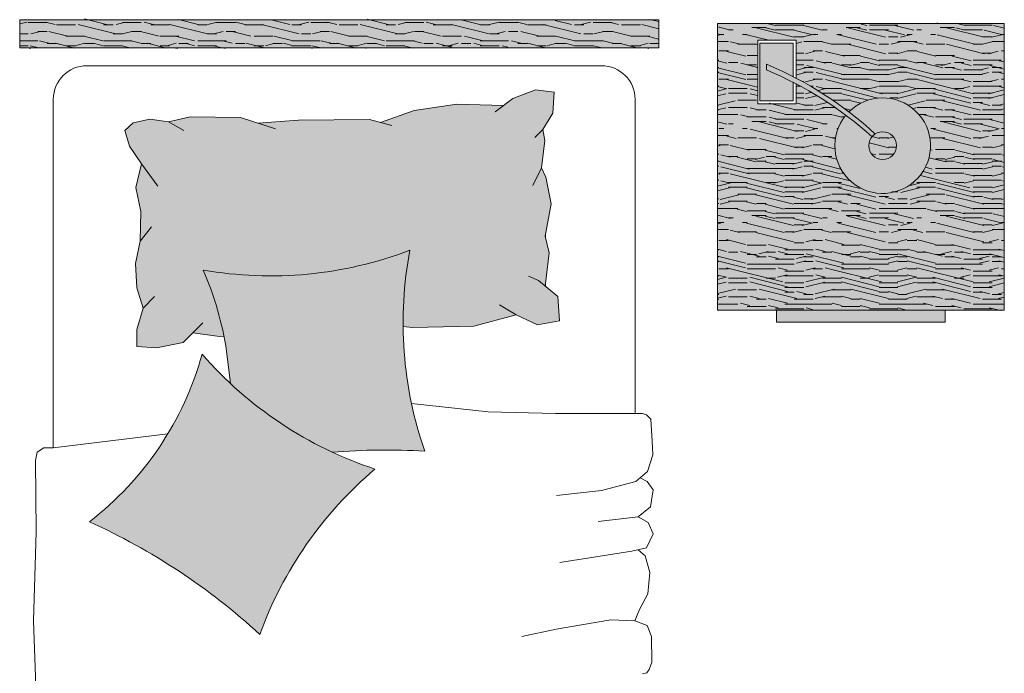
# Model space of a CAD drawing. Units: inches. Extents: x 1994 to 3075, y 3517 to 3950.
# Tile 19 of 58: x 1994.71013 to 1994.76776, y 3553.27657 to 3553.31483. Entities that reach past the tile are written whole.
import ezdxf

# ---------------------------------------------------------------- set-up
doc = ezdxf.new("R2010")
doc.units = ezdxf.units.IN
doc.layers.add('A-FURN-REFR', color=8, linetype='Continuous', lineweight=13)
doc.layers.add('A-FURN-REFR-PATT', color=8, linetype='Continuous', lineweight=13)

msp = doc.modelspace()

# ---------------------------------------------------------------- hatches: boundary and pattern name
at = {"layer": 'A-FURN-REFR-PATT'}
for points in [[(1994.74752711248, 3553.314834833183), (1994.710125537677, 3553.314834833183), (1994.710125537677, 3553.313186285147), (1994.74752711248, 3553.313186285147)], [(1994.755400221191, 3553.313454285159), (1994.753453346297, 3553.313454285159), (1994.753453346297, 3553.310087285902), (1994.755400221191, 3553.310087285902), (1994.755400221191, 3553.311165699976, 0.0198106445216732), (1994.753838065744, 3553.311892743406), (1994.753838065744, 3553.312223669301, -0.0198106445216994), (1994.755400221191, 3553.311496625872), (1994.755400221191, 3553.311503507754)]]:
    msp.add_hatch(color=256, dxfattribs=at).paths.add_polyline_path(points)
h = msp.add_hatch(dxfattribs=at)
h.set_pattern_fill('LEGNO1', color=256, scale=0.005511811023622, style=0, pattern_type=2)
h.set_pattern_definition([(0, (2000.356371596277, 3548.921636491977), (0, 0.005511811023622), [0.0011023622047244, -0.0016535433070866, 0.0005511811023622, -0.0022047244094488]), (0, (2000.360229863994, 3548.921774287253), (0, 0.005511811023622), [0.0011023622047244, -0.0044094488188976]), (0, (2000.359678682892, 3548.922049877804), (0, 0.005511811023622), [0.0005511811023622, -0.0049606299212598]), (0, (2000.356647186829, 3548.92218767308), (0, 0.005511811023622), [0.0002755905511811, -0.0038582677165354, 0.0002755905511811, -0.0011023622047244]), (0, (2000.358576320687, 3548.922463263631), (0, 0.005511811023622), [0.0011023622047244, -0.0016535433070866, 0.0002755905511811, -0.0024803149606299]), (0, (2000.357198367931, 3548.922601058907), (0, 0.005511811023622), [0.0008267716535433, -0.0046850393700787]), (0, (2000.358576320687, 3548.922738854182), (0, 0.005511811023622), [0.0016535433070866, -0.0038582677165354]), (0, (2000.356922777379, 3548.922876649458), (0, 0.005511811023622), [0.0011023622047244, -0.0044094488188976]), (0, (2000.35912750179, 3548.923014444734), (0, 0.005511811023622), [0.002755905511811, -0.002755905511811]), (0, (2000.357473958482, 3548.923290035285), (0, 0.005511811023622), [0.0005511811023622, -0.0016535433070866, 0.0011023622047244, -0.0022047244094488]), (0, (2000.361332226199, 3548.923427830561), (0, 0.005511811023622), [0.0011023622047244, -0.0044094488188976]), (0, (2000.360229863994, 3548.923565625836), (0, 0.005511811023622), [0.0005511811023622, -0.0049606299212598]), (0, (2000.35912750179, 3548.923703421111), (0, 0.005511811023622), [0.0005511811023622, -0.0049606299212598]), (0, (2000.356371596277, 3548.923841216387), (0, 0.005511811023622), [0.0011023622047244, -0.0044094488188976]), (0, (2000.35912750179, 3548.923979011662), (0, 0.005511811023622), [0.0011023622047244, -0.0044094488188976]), (0, (2000.35912750179, 3548.924254602213), (0, 0.005511811023622), [0.0011023622047244, -0.0011023622047244, 0.0011023622047244, -0.0022047244094488]), (0, (2000.358025139584, 3548.924530192765), (0, 0.005511811023622), [0.0005511811023622, -0.002755905511811, 0.0011023622047244, -0.0011023622047244]), (0, (2000.35912750179, 3548.92466798804), (0, 0.005511811023622), [0.0016535433070866, -0.0038582677165354]), (0, (2000.35912750179, 3548.924943578592), (0, 0.005511811023622), [0.0011023622047244, -0.0044094488188976]), (0, (2000.356922777379, 3548.925081373867), (0, 0.005511811023622), [0.0016535433070866, -0.0022047244094488, 0.0005511811023622, -0.0011023622047244]), (0, (2000.356922777379, 3548.925356964419), (0, 0.005511811023622), [0.002755905511811, -0.002755905511811]), (0, (2000.360229863994, 3548.925494759694), (0, 0.005511811023622), [0.0005511811023622, -0.0049606299212598]), (0, (2000.358576320687, 3548.92563255497), (0, 0.005511811023622), [0.0011023622047244, -0.0044094488188976]), (0, (2000.357473958482, 3548.925770350245), (0, 0.005511811023622), [0.0005511811023622, -0.0022047244094488, 0.0005511811023622, -0.0022047244094488]), (0, (2000.356922777379, 3548.925908145521), (0, 0.005511811023622), [0.0005511811023622, -0.0016535433070866, 0.0011023622047244, -0.0022047244094488]), (0, (2000.358025139584, 3548.926045940796), (0, 0.005511811023622), [0.0005511811023622, -0.002755905511811, 0.0005511811023622, -0.0016535433070866]), (0, (2000.35912750179, 3548.926183736072), (0, 0.005511811023622), [0.0016535433070866, -0.0038582677165354]), (0, (2000.356922777379, 3548.926459326623), (0, 0.005511811023622), [0.0011023622047244, -0.0044094488188976]), (0, (2000.359678682892, 3548.926597121898), (0, 0.005511811023622), [0.0005511811023622, -0.0049606299212598]), (0, (2000.360781045096, 3548.926734917174), (0, 0.005511811023622), [0.0005511811023622, -0.0049606299212598]), (14.03624347, (2000.360229863994, 3548.922049877804), (0.0055118110234648, -2.016e-13), [0.0005677165354331, -0.0221580619543307]), (14.03624347, (2000.360781045096, 3548.923290035285), (0.0055118110234648, -2.016e-13), [0.0005677165354331, -0.0221580619543307]), (14.03624347, (2000.360229863994, 3548.926597121898), (0.0055118110234648, -2.016e-13), [0.0005677165354331, -0.0221580619543307]), (14.03624347, (2000.358576320687, 3548.924530192765), (0.0055118110234648, -2.016e-13), [0.0005677165354331, -0.0221580619543307]), (14.03624347, (2000.359678682892, 3548.925356964419), (0.0055118110234648, -2.016e-13), [0.0005677165354331, -0.0221580619543307]), (14.03624347, (2000.360229863994, 3548.924943578592), (0.0055118110234648, -2.016e-13), [0.0005677165354331, -0.0221580619543307]), (14.03624347, (2000.357473958482, 3548.925908145521), (0.0055118110234648, -2.016e-13), [0.0005677165354331, -0.0221580619543307]), (14.03624347, (2000.359678682892, 3548.92563255497), (0.0055118110234648, -2.016e-13), [0.0005677165354331, -0.0221580619543307]), (14.03624347, (2000.360781045096, 3548.923565625836), (0.0055118110234648, -2.016e-13), [0.0011354330708661, -0.0215903454188977]), (14.03624347, (2000.360229863994, 3548.923979011662), (0.0055118110234648, -2.016e-13), [0.0011354330708661, -0.0215903454188977]), (14.03624347, (2000.360229863994, 3548.924254602213), (0.0055118110234648, -2.016e-13), [0.0011354330708661, -0.0215903454188977]), (165.96375653, (2000.358576320687, 3548.922463263631), (-0.0055118110234648, -2.016e-13), [0.0005677165354331, -0.0011354330708661, 0.0005677165354331, -0.0204549123480315]), (165.96375653, (2000.357473958482, 3548.923290035285), (-0.0055118110234648, -2.016e-13), [0.0005677165354331, -0.0221580619543307]), (165.96375653, (2000.357473958482, 3548.925770350245), (-0.0055118110234648, -2.016e-13), [0.0011354330708661, -0.0215903454188977]), (194.03624347, (2000.360229863994, 3548.921774287253), (-0.0055118110234648, 2.016e-13), [0.0005677165354331, -0.0221580619543307]), (345.96375653, (2000.361332226199, 3548.921774287253), (0.0055118110234648, 2.016e-13), [0.0005677165354331, -0.0221580619543307]), (345.96375653, (2000.359678682892, 3548.923703421111), (0.0055118110234648, 2.016e-13), [0.0005677165354331, -0.0221580619543307]), (345.96375653, (2000.360781045096, 3548.92466798804), (0.0055118110234648, 2.016e-13), [0.0005677165354331, -0.0221580619543307]), (345.96375653, (2000.358576320687, 3548.925081373867), (0.0055118110234648, 2.016e-13), [0.0005677165354331, -0.0221580619543307]), (345.96375653, (2000.358025139584, 3548.925770350245), (0.0055118110234648, 2.016e-13), [0.0005677165354331, -0.0221580619543307]), (345.96375653, (2000.358576320687, 3548.926045940796), (0.0055118110234648, 2.016e-13), [0.0005677165354331, -0.0221580619543307]), (345.96375653, (2000.358576320687, 3548.925081373867), (0.0055118110234648, 2.016e-13), [0.0005677165354331, -0.0221580619543307]), (345.96375653, (2000.360229863994, 3548.925908145521), (0.0055118110234648, 2.016e-13), [0.0022708661417323, -0.0204549123480315]), (345.96375653, (2000.356922777379, 3548.92218767308), (0.0055118110234648, 2.016e-13), [0.0022708661417323, -0.0204549123480315]), (345.96375653, (2000.357473958482, 3548.922601058907), (0.0055118110234648, 2.016e-13), [0.0022708661417323, -0.0204549123480315]), (345.96375653, (2000.358025139584, 3548.922876649458), (0.0055118110234648, 2.016e-13), [0.0005677165354331, -0.0011354330708661, 0.0011354330708661, -0.0198871958125984]), (345.96375653, (2000.358025139584, 3548.923290035285), (0.0055118110234648, 2.016e-13), [0.0011354330708661, -0.0011354330708661, 0.0011354330708661, -0.0193194792771654]), (345.96375653, (2000.357473958482, 3548.923841216387), (0.0055118110234648, 2.016e-13), [0.0022708661417323, -0.0204549123480315]), (345.96375653, (2000.356922777379, 3548.924254602213), (0.0055118110234648, 2.016e-13), [0.0022708661417323, -0.0204549123480315]), (345.96375653, (2000.356922777379, 3548.924530192765), (0.0055118110234648, 2.016e-13), [0.0022708661417323, -0.0204549123480315]), (345.96375653, (2000.360781045096, 3548.926183736072), (0.0055118110234648, 2.016e-13), [0.0005677165354331, -0.0221580619543307]), (345.9637675300001, (2000.361332226199, 3548.926734917174), (0.0055118110234647, 1.0583933e-09), [0.0011354330708661, -0.0215903454188977]), (345.9637675300001, (2000.358025139584, 3548.926459326623), (0.0055118110234647, 1.0583933e-09), [0.0011354330708661, -0.0215903454188977]), (345.96375753, (2000.357473958482, 3548.921636491977), (0.0055118110234648, 9.64008e-11), [0.0022708661417323, -0.0204549123480315]), (345.96375753, (2000.360781045096, 3548.925494759694), (0.0055118110234648, 9.64008e-11), [0.0017031496062992, -0.0210226288834646]), (345.96375753, (2000.361332226199, 3548.925081373867), (0.0055118110234648, 9.64008e-11), [0.0034062992125984, -0.0193194792771654])])
h.paths.add_polyline_path([(1994.74752711248, 3553.314834833183), (1994.710125537677, 3553.314834833183), (1994.710125537677, 3553.313186285147), (1994.74752711248, 3553.313186285147)])
h = msp.add_hatch(color=256, dxfattribs=at)
h.paths.add_polyline_path([(1994.76775604609, 3553.314620330361), (1994.750973187446, 3553.314620330361), (1994.750973187446, 3553.297837471717), (1994.76775604609, 3553.297837471717)])
h.paths.add_polyline_path([(1994.758479567912, 3553.309240305821, 0.0395152736214826), (1994.755577209817, 3553.311073603386), (1994.755577209817, 3553.309910077288), (1994.753320605166, 3553.309910077288), (1994.753320605166, 3553.313631493773), (1994.755577209817, 3553.313631493773), (1994.755577209817, 3553.311404529282, -0.042086183498597), (1994.758657689699, 3553.309436525341, -42.19598506439468)], flags=16)
h.paths.add_polyline_path([(1994.759827418463, 3553.30746046484, -1), (1994.761447352029, 3553.30746046484, -1)], flags=0)
h = msp.add_hatch(dxfattribs=at)
h.set_pattern_fill('LEGNO1', color=256, scale=0.005511811023622, style=0, pattern_type=2)
h.set_pattern_definition([(0, (2000.776563016131, 3549.493707209018), (0, 0.005511811023622), [0.0011023622047244, -0.0016535433070866, 0.0005511811023622, -0.0022047244094488]), (0, (2000.780421283847, 3549.493845004293), (0, 0.005511811023622), [0.0011023622047244, -0.0044094488188976]), (0, (2000.779870102745, 3549.494120594844), (0, 0.005511811023622), [0.0005511811023622, -0.0049606299212598]), (0, (2000.776838606682, 3549.49425839012), (0, 0.005511811023622), [0.0002755905511811, -0.0038582677165354, 0.0002755905511811, -0.0011023622047244]), (0, (2000.77876774054, 3549.494533980671), (0, 0.005511811023622), [0.0011023622047244, -0.0016535433070866, 0.0002755905511811, -0.0024803149606299]), (0, (2000.777389787784, 3549.494671775947), (0, 0.005511811023622), [0.0008267716535433, -0.0046850393700787]), (0, (2000.77876774054, 3549.494809571223), (0, 0.005511811023622), [0.0016535433070866, -0.0038582677165354]), (0, (2000.777114197233, 3549.494947366498), (0, 0.005511811023622), [0.0011023622047244, -0.0044094488188976]), (0, (2000.779318921642, 3549.495085161774), (0, 0.005511811023622), [0.002755905511811, -0.002755905511811]), (0, (2000.777665378335, 3549.495360752325), (0, 0.005511811023622), [0.0005511811023622, -0.0016535433070866, 0.0011023622047244, -0.0022047244094488]), (0, (2000.781523646052, 3549.4954985476), (0, 0.005511811023622), [0.0011023622047244, -0.0044094488188976]), (0, (2000.780421283847, 3549.495636342876), (0, 0.005511811023622), [0.0005511811023622, -0.0049606299212598]), (0, (2000.779318921642, 3549.495774138151), (0, 0.005511811023622), [0.0005511811023622, -0.0049606299212598]), (0, (2000.776563016131, 3549.495911933428), (0, 0.005511811023622), [0.0011023622047244, -0.0044094488188976]), (0, (2000.779318921642, 3549.496049728702), (0, 0.005511811023622), [0.0011023622047244, -0.0044094488188976]), (0, (2000.779318921642, 3549.496325319254), (0, 0.005511811023622), [0.0011023622047244, -0.0011023622047244, 0.0011023622047244, -0.0022047244094488]), (0, (2000.778216559438, 3549.496600909805), (0, 0.005511811023622), [0.0005511811023622, -0.002755905511811, 0.0011023622047244, -0.0011023622047244]), (0, (2000.779318921642, 3549.496738705081), (0, 0.005511811023622), [0.0016535433070866, -0.0038582677165354]), (0, (2000.779318921642, 3549.497014295632), (0, 0.005511811023622), [0.0011023622047244, -0.0044094488188976]), (0, (2000.777114197233, 3549.497152090907), (0, 0.005511811023622), [0.0016535433070866, -0.0022047244094488, 0.0005511811023622, -0.0011023622047244]), (0, (2000.777114197233, 3549.497427681459), (0, 0.005511811023622), [0.002755905511811, -0.002755905511811]), (0, (2000.780421283847, 3549.497565476734), (0, 0.005511811023622), [0.0005511811023622, -0.0049606299212598]), (0, (2000.77876774054, 3549.49770327201), (0, 0.005511811023622), [0.0011023622047244, -0.0044094488188976]), (0, (2000.777665378335, 3549.497841067285), (0, 0.005511811023622), [0.0005511811023622, -0.0022047244094488, 0.0005511811023622, -0.0022047244094488]), (0, (2000.777114197233, 3549.497978862561), (0, 0.005511811023622), [0.0005511811023622, -0.0016535433070866, 0.0011023622047244, -0.0022047244094488]), (0, (2000.778216559438, 3549.498116657836), (0, 0.005511811023622), [0.0005511811023622, -0.002755905511811, 0.0005511811023622, -0.0016535433070866]), (0, (2000.779318921642, 3549.498254453112), (0, 0.005511811023622), [0.0016535433070866, -0.0038582677165354]), (0, (2000.777114197233, 3549.498530043663), (0, 0.005511811023622), [0.0011023622047244, -0.0044094488188976]), (0, (2000.779870102745, 3549.498667838939), (0, 0.005511811023622), [0.0005511811023622, -0.0049606299212598]), (0, (2000.78097246495, 3549.498805634215), (0, 0.005511811023622), [0.0005511811023622, -0.0049606299212598]), (14.03624347, (2000.780421283847, 3549.494120594844), (0.0055118110234648, -2.016e-13), [0.0005677165354331, -0.0221580619543307]), (14.03624347, (2000.78097246495, 3549.495360752325), (0.0055118110234648, -2.016e-13), [0.0005677165354331, -0.0221580619543307]), (14.03624347, (2000.780421283847, 3549.498667838939), (0.0055118110234648, -2.016e-13), [0.0005677165354331, -0.0221580619543307]), (14.03624347, (2000.77876774054, 3549.496600909805), (0.0055118110234648, -2.016e-13), [0.0005677165354331, -0.0221580619543307]), (14.03624347, (2000.779870102745, 3549.497427681459), (0.0055118110234648, -2.016e-13), [0.0005677165354331, -0.0221580619543307]), (14.03624347, (2000.780421283847, 3549.497014295632), (0.0055118110234648, -2.016e-13), [0.0005677165354331, -0.0221580619543307]), (14.03624347, (2000.777665378335, 3549.497978862561), (0.0055118110234648, -2.016e-13), [0.0005677165354331, -0.0221580619543307]), (14.03624347, (2000.779870102745, 3549.49770327201), (0.0055118110234648, -2.016e-13), [0.0005677165354331, -0.0221580619543307]), (14.03624347, (2000.78097246495, 3549.495636342876), (0.0055118110234648, -2.016e-13), [0.0011354330708661, -0.0215903454188977]), (14.03624347, (2000.780421283847, 3549.496049728702), (0.0055118110234648, -2.016e-13), [0.0011354330708661, -0.0215903454188977]), (14.03624347, (2000.780421283847, 3549.496325319254), (0.0055118110234648, -2.016e-13), [0.0011354330708661, -0.0215903454188977]), (165.96375653, (2000.77876774054, 3549.494533980671), (-0.0055118110234648, -2.016e-13), [0.0005677165354331, -0.0011354330708661, 0.0005677165354331, -0.0204549123480315]), (165.96375653, (2000.777665378335, 3549.495360752325), (-0.0055118110234648, -2.016e-13), [0.0005677165354331, -0.0221580619543307]), (165.96375653, (2000.777665378335, 3549.497841067285), (-0.0055118110234648, -2.016e-13), [0.0011354330708661, -0.0215903454188977]), (194.03624347, (2000.780421283847, 3549.493845004293), (-0.0055118110234648, 2.016e-13), [0.0005677165354331, -0.0221580619543307]), (345.96375653, (2000.781523646052, 3549.493845004293), (0.0055118110234648, 2.016e-13), [0.0005677165354331, -0.0221580619543307]), (345.96375653, (2000.779870102745, 3549.495774138151), (0.0055118110234648, 2.016e-13), [0.0005677165354331, -0.0221580619543307]), (345.96375653, (2000.78097246495, 3549.496738705081), (0.0055118110234648, 2.016e-13), [0.0005677165354331, -0.0221580619543307]), (345.96375653, (2000.77876774054, 3549.497152090907), (0.0055118110234648, 2.016e-13), [0.0005677165354331, -0.0221580619543307]), (345.96375653, (2000.778216559438, 3549.497841067285), (0.0055118110234648, 2.016e-13), [0.0005677165354331, -0.0221580619543307]), (345.96375653, (2000.77876774054, 3549.498116657836), (0.0055118110234648, 2.016e-13), [0.0005677165354331, -0.0221580619543307]), (345.96375653, (2000.77876774054, 3549.497152090907), (0.0055118110234648, 2.016e-13), [0.0005677165354331, -0.0221580619543307]), (345.96375653, (2000.780421283847, 3549.497978862561), (0.0055118110234648, 2.016e-13), [0.0022708661417323, -0.0204549123480315]), (345.96375653, (2000.777114197233, 3549.49425839012), (0.0055118110234648, 2.016e-13), [0.0022708661417323, -0.0204549123480315]), (345.96375653, (2000.777665378335, 3549.494671775947), (0.0055118110234648, 2.016e-13), [0.0022708661417323, -0.0204549123480315]), (345.96375653, (2000.778216559438, 3549.494947366498), (0.0055118110234648, 2.016e-13), [0.0005677165354331, -0.0011354330708661, 0.0011354330708661, -0.0198871958125984]), (345.96375653, (2000.778216559438, 3549.495360752325), (0.0055118110234648, 2.016e-13), [0.0011354330708661, -0.0011354330708661, 0.0011354330708661, -0.0193194792771654]), (345.96375653, (2000.777665378335, 3549.495911933428), (0.0055118110234648, 2.016e-13), [0.0022708661417323, -0.0204549123480315]), (345.96375653, (2000.777114197233, 3549.496325319254), (0.0055118110234648, 2.016e-13), [0.0022708661417323, -0.0204549123480315]), (345.96375653, (2000.777114197233, 3549.496600909805), (0.0055118110234648, 2.016e-13), [0.0022708661417323, -0.0204549123480315]), (345.96375653, (2000.78097246495, 3549.498254453112), (0.0055118110234648, 2.016e-13), [0.0005677165354331, -0.0221580619543307]), (345.9637675300001, (2000.781523646052, 3549.498805634215), (0.0055118110234647, 1.0583933e-09), [0.0011354330708661, -0.0215903454188977]), (345.9637675300001, (2000.778216559438, 3549.498530043663), (0.0055118110234647, 1.0583933e-09), [0.0011354330708661, -0.0215903454188977]), (345.96375753, (2000.777665378335, 3549.493707209018), (0.0055118110234648, 9.64008e-11), [0.0022708661417323, -0.0204549123480315]), (345.96375753, (2000.78097246495, 3549.497565476734), (0.0055118110234648, 9.64008e-11), [0.0017031496062992, -0.0210226288834646]), (345.96375753, (2000.781523646052, 3549.497152090907), (0.0055118110234648, 9.64008e-11), [0.0034062992125984, -0.0193194792771654])])
h.paths.add_polyline_path([(1994.76775604609, 3553.314620330361), (1994.750973187446, 3553.314620330361), (1994.750973187446, 3553.297837471717), (1994.76775604609, 3553.297837471717)])
h.paths.add_polyline_path([(1994.753320605166, 3553.309910077288), (1994.753320605166, 3553.313631493773), (1994.755577209817, 3553.313631493773), (1994.755577209817, 3553.311404529282, -0.042086183498597), (1994.758657689699, 3553.309436525341, -42.19598506432865), (1994.758479567912, 3553.309240305821, 0.0395152736214861), (1994.755577209817, 3553.311073603386), (1994.755577209817, 3553.309910077288)], flags=16)
h.paths.add_polyline_path([(1994.759827418463, 3553.30746046484, -1), (1994.761447352029, 3553.30746046484, -1)], flags=0)
h = msp.add_hatch(color=256, dxfattribs=at)
h.dxf.hatch_style = 1
h.set_gradient(color1=(167, 169, 175), one_color=1, tint=1)
h.paths.add_polyline_path([(1994.753838065744, 3553.311892743406), (1994.753838065744, 3553.312223669301, -0.0875286051314429), (1994.76019873732, 3553.308141371726, 0.0763380806476787), (1994.760014634205, 3553.307978371522, 0.0846435149619904)])
h = msp.add_hatch(color=256, dxfattribs=at)
h.set_gradient(color1=(223, 184, 155), color2=(248, 239, 232), one_color=1, tint=0.9399999976158142, name='SPHERICAL')
edge = h.paths.add_edge_path()
edge.add_ellipse((1994.724813374119, 3553.322745777475), major_axis=(-0.0162394621936465, 0.0161586354510627), ratio=0.9999999999999754, start_angle=124.93165070209781, end_angle=155.6980503708569, ccw=False)
edge.add_ellipse((1994.703806775848, 3553.292701605456), major_axis=(0.0131369998350938, 0.013202712122942), ratio=0.9999999999990169, start_angle=326.0032218548852, end_angle=338.5294090826841, ccw=False)
edge.add_line((1994.722080502796, 3553.296302060358), (1994.721824171691, 3553.29628022039))
edge.add_line((1994.721824171691, 3553.29628022039), (1994.720265573822, 3553.296506067916))
edge.add_line((1994.720265573822, 3553.296506067916), (1994.719692777913, 3553.295935777522))
edge.add_line((1994.719692777912, 3553.295935777522), (1994.718133224533, 3553.295626048687))
edge.add_line((1994.718133224533, 3553.295626048687), (1994.716980872298, 3553.29569946425))
edge.add_line((1994.716980872298, 3553.29569946425), (1994.716991652343, 3553.296703707926))
edge.add_line((1994.716991652343, 3553.296703707926), (1994.717346825471, 3553.297943913479))
edge.add_line((1994.717346825471, 3553.29794391348), (1994.716987198101, 3553.299140726493))
edge.add_line((1994.716987198101, 3553.299140726492), (1994.716900483803, 3553.300569161474))
edge.add_line((1994.716900483803, 3553.300569161474), (1994.717179841152, 3553.301876449751))
edge.add_line((1994.717179841153, 3553.301876449751), (1994.717218744079, 3553.303599250499))
edge.add_line((1994.717218744079, 3553.303599250499), (1994.716917589632, 3553.305014667718))
edge.add_line((1994.716917589632, 3553.305014667718), (1994.717264091322, 3553.3063977169))
edge.add_line((1994.717264091322, 3553.3063977169), (1994.71655573514, 3553.307429990013))
edge.add_line((1994.71655573514, 3553.307429990013), (1994.716284930695, 3553.308345455022))
edge.add_line((1994.716284930695, 3553.308345455022), (1994.716759276751, 3553.30880436036))
edge.add_line((1994.716759276751, 3553.308804360361), (1994.717751326011, 3553.309007953546))
edge.add_line((1994.717751326011, 3553.309007953546), (1994.718836533334, 3553.308858777043))
edge.add_line((1994.718836533334, 3553.308858777043), (1994.720110166515, 3553.309151148862))
edge.add_line((1994.720110166515, 3553.309151148862), (1994.723053855134, 3553.309114792965))
edge.add_line((1994.723053855134, 3553.309114792965), (1994.724070921565, 3553.308785153716))
edge.add_line((1994.724070921565, 3553.308785153716), (1994.72643509492, 3553.308961628929))
edge.add_line((1994.72643509492, 3553.308961628929), (1994.730593944388, 3553.308999040351))
edge.add_line((1994.730593944387, 3553.308999040351), (1994.731250378423, 3553.308823799849))
edge.add_line((1994.731250378423, 3553.308823799849), (1994.733217026507, 3553.309516701592))
edge.add_line((1994.733217026506, 3553.309516701592), (1994.735705820534, 3553.309882840731))
edge.add_line((1994.735705820534, 3553.309882840731), (1994.738447054648, 3553.30981764357))
edge.add_line((1994.738447054649, 3553.30981764357), (1994.738985230838, 3553.310225289685))
edge.add_line((1994.738985230838, 3553.310225289685), (1994.740317336921, 3553.310736266038))
edge.add_line((1994.740317336921, 3553.310736266038), (1994.741402544245, 3553.310587089535))
edge.add_line((1994.741402544245, 3553.310587089535), (1994.741333291296, 3553.309364241325))
edge.add_line((1994.741333291296, 3553.309364241325), (1994.740746335734, 3553.308396704976))
edge.add_line((1994.740746335734, 3553.308396704975), (1994.740856837224, 3553.307758248389))
edge.add_line((1994.740856837224, 3553.307758248389), (1994.74066630276, 3553.306169612763))
edge.add_line((1994.74066630276, 3553.306169612762), (1994.740915428641, 3553.305611256336))
edge.add_line((1994.740915428641, 3553.305611256336), (1994.741225254526, 3553.304052995487))
edge.add_line((1994.741225254526, 3553.304052995488), (1994.740888795057, 3553.302153237223))
edge.add_line((1994.740888795058, 3553.302153237223), (1994.741112762962, 3553.301178767854))
edge.add_line((1994.741112762962, 3553.301178767853), (1994.740891792206, 3553.299235319621))
edge.add_line((1994.740891792206, 3553.299235319622), (1994.741626248971, 3553.298629280765))
edge.add_line((1994.741626248971, 3553.298629280765), (1994.741712963269, 3553.297200845783))
edge.add_line((1994.741712963269, 3553.297200845783), (1994.740434993809, 3553.296979895581))
edge.add_line((1994.740434993809, 3553.296979895581), (1994.739180812092, 3553.297548924135))
edge.add_line((1994.739180812092, 3553.297548924135), (1994.73670936092, 3553.296897098066))
edge.add_line((1994.73670936092, 3553.296897098066), (1994.733126688151, 3553.296822978733))
edge.add_line((1994.733126688151, 3553.296822978733), (1994.73256889776, 3553.29686572429))
edge.add_ellipse((1994.755545523121, 3553.297088097322), major_axis=(0.0162071033392254, 0.0162881725219294), ratio=0.9999999999997861, start_angle=124.2042415032482, end_angle=135.411563179048, ccw=False)
h = msp.add_hatch(color=256, dxfattribs=at)
h.dxf.hatch_style = 1
h.set_gradient(color1=(37, 53, 157), color2=(142, 207, 230), tint=1, name='SPHERICAL')
h.paths.add_polyline_path([(1994.760637385246, 3553.308270431623, 0.1440580758931676), (1994.76019873732, 3553.308141371726, 0.0231477939795123), (1994.758657689699, 3553.309436525341, -42.19598506439846), (1994.758479567912, 3553.309240305821, -0.0228504078660832), (1994.760014634205, 3553.307978371522, 0.6355278128427492), (1994.760637385246, 3553.306650498058, 1)])
h = msp.add_hatch(color=256, dxfattribs=at)
h.dxf.hatch_style = 1
h.set_gradient(color1=(37, 40, 142), tint=1, name='INVSPHERICAL')
h.paths.add_polyline_path([(1994.760637385246, 3553.306650498058, -1), (1994.760637385246, 3553.308270431623, -1)])
h = msp.add_hatch(color=256, dxfattribs=at)
h.set_gradient(color1=(216, 161, 105), color2=(246, 232, 219), one_color=1, tint=0.9100000262260437, name='SPHERICAL')
edge = h.paths.add_edge_path()
edge.add_ellipse((1994.738091277294, 3553.310284112182), major_axis=(-0.0162394621936562, 0.0161586354510724), ratio=0.9999999999995159, start_angle=91.86790391008537, end_angle=109.9005060978115, ccw=False)
edge.add_line((1994.722470558145, 3553.293526583568), (1994.722230916878, 3553.295429864856))
edge.add_ellipse((1994.703806775848, 3553.292701605456), major_axis=(-0.0132027121229715, 0.0131369998351231), ratio=0.9999999999985743, start_angle=233.2802454111125, end_angle=248.5294090826748)
edge.add_ellipse((1994.724813374119, 3553.322745777475), major_axis=(-0.0162394621936476, 0.0161586354510638), ratio=0.9999999999999643, start_angle=124.9316507020978, end_angle=155.6980503708595)
edge.add_ellipse((1994.755545523121, 3553.297088097322), major_axis=(0.0162071033392156, 0.0162881725219195), ratio=0.9999999999999907, start_angle=124.2042415032435, end_angle=153.9185959955232)
edge.add_line((1994.733827726711, 3553.289583959675), (1994.733816342417, 3553.289572575381))
edge.add_ellipse((1994.731531269729, 3553.251646479053), major_axis=(-0.026933374560409, 0.0267993222804413), ratio=0.9999999999999866, start_angle=-48.5908820798409, end_angle=-40.45389875014118)
h = msp.add_hatch(color=256, dxfattribs=at)
h.set_gradient(color1=(158, 155, 166), rotation=89.99999999999996, one_color=1, tint=1)
h.paths.add_polyline_path([(1994.764302349481, 3553.297837471717), (1994.754426884055, 3553.297837471717), (1994.754426884055, 3553.297131545392), (1994.764302349481, 3553.297131545392)])
h = msp.add_hatch(color=256, dxfattribs=at)
h.set_gradient(color1=(216, 161, 105), color2=(246, 232, 219), one_color=1, tint=0.9100000262260437, name='SPHERICAL')
edge = h.paths.add_edge_path()
edge.add_ellipse((1994.738091277294, 3553.310284112182), major_axis=(-0.0162394621936485, 0.0161586354510647), ratio=0.9999999999999784, start_angle=85.852665878386, end_angle=116.6190655471458)
edge.add_ellipse((1994.745773584699, 3553.270993353904), major_axis=(0.016207103339218, 0.0162881725219219), ratio=0.9999999999998035, start_angle=85.12525667954132, end_angle=114.8721443105295)
edge.add_ellipse((1994.698485863071, 3553.250856412228), major_axis=(-0.0269333745604207, 0.026799322280453), ratio=0.9999999999996999, start_angle=-87.69350806299315, end_angle=-69.58500463641445)
edge.add_ellipse((1994.702844744636, 3553.300203865216), major_axis=(0.0131369998350991, 0.0132027121229474), ratio=0.9999999999998083, start_angle=262.4507864490607, end_angle=299.4504242589634)

# ---------------------------------------------------------------- linework, layer by layer
at = {"layer": 'A-FURN-REFR'}
for p, q in [((1994.710125537677, 3553.313186285147), (1994.710125537677, 3553.314834833183)), ((1994.74752711248, 3553.314834833183), (1994.710125537677, 3553.314834833183)), ((1994.74752711248, 3553.313186285147), (1994.74752711248, 3553.314834833183)), ((1994.76775604609, 3553.314620330361), (1994.750973187446, 3553.314620330361)), ((1994.750973187446, 3553.314620330361), (1994.750973187446, 3553.297837471717)), ((1994.76775604609, 3553.297837471717), (1994.76775604609, 3553.314620330361)), ((1994.710125537677, 3553.313186285147), (1994.74752711248, 3553.313186285147)), ((1994.753838065744, 3553.312223669301), (1994.753838065744, 3553.311892743406)), ((1994.714062545551, 3553.312143118972), (1994.721377585873, 3553.312143118972)), ((1994.721377585873, 3553.312143118972), (1994.744176183505, 3553.312143118972)), ((1994.740317336921, 3553.310736266038), (1994.738985230838, 3553.310225289685)), ((1994.741402544245, 3553.310587089535), (1994.740317336921, 3553.310736266038)), ((1994.741333291296, 3553.309364241325), (1994.741402544245, 3553.310587089535)), ((1994.712094041614, 3553.289770163587), (1994.712094041614, 3553.310174615035)), ((1994.733217026506, 3553.309516701592), (1994.735705820534, 3553.309882840731)), ((1994.735705820534, 3553.309882840731), (1994.738447054649, 3553.30981764357)), ((1994.738985230838, 3553.310225289685), (1994.737956387239, 3553.309445983383)), ((1994.746144687441, 3553.29505004844), (1994.746144687441, 3553.310174615035)), ((1994.731250378423, 3553.308823799849), (1994.733217026506, 3553.309516701592)), ((1994.740746335734, 3553.308396704975), (1994.741333291296, 3553.309364241325)), ((1994.716759276751, 3553.308804360361), (1994.716284930695, 3553.308345455022)), ((1994.717751326011, 3553.309007953546), (1994.716759276751, 3553.308804360361)), ((1994.718836533334, 3553.308858777043), (1994.717751326011, 3553.309007953546)), ((1994.718836533334, 3553.308858777043), (1994.720110166515, 3553.309151148862)), ((1994.718836533334, 3553.308858777043), (1994.719728979664, 3553.308339473903)), ((1994.720110166515, 3553.309151148862), (1994.723053855134, 3553.309114792965)), ((1994.723053855134, 3553.309114792965), (1994.725102988837, 3553.308450652576)), ((1994.724070921565, 3553.308785153716), (1994.72643509492, 3553.308961628929)), ((1994.72643509492, 3553.308961628929), (1994.730593944387, 3553.308999040351)), ((1994.730593944387, 3553.308999040351), (1994.731906599007, 3553.30864861633)), ((1994.716284930695, 3553.308345455022), (1994.71655573514, 3553.307429990013)), ((1994.740271989678, 3553.307937799637), (1994.740746335734, 3553.308396704975)), ((1994.740856837224, 3553.307758248389), (1994.740746335734, 3553.308396704975)), ((1994.74066630276, 3553.306169612762), (1994.740856837224, 3553.307758248389)), ((1994.71655573514, 3553.307429990013), (1994.717264091322, 3553.3063977169)), ((1994.717264091322, 3553.3063977169), (1994.716917589632, 3553.305014667718)), ((1994.717264091322, 3553.3063977169), (1994.718204229958, 3553.305092774257)), ((1994.740155162385, 3553.30513499398), (1994.74066630276, 3553.306169612762)), ((1994.740915428641, 3553.305611256336), (1994.74066630276, 3553.306169612762)), ((1994.741225254526, 3553.304052995488), (1994.740915428641, 3553.305611256336)), ((1994.716917589632, 3553.305014667718), (1994.717218744079, 3553.303599250499)), ((1994.717218744079, 3553.303599250499), (1994.717179841153, 3553.301876449751)), ((1994.740888795058, 3553.302153237223), (1994.741225254526, 3553.304052995488)), ((1994.717846948793, 3553.302705481434), (1994.717179841153, 3553.301876449751)), ((1994.717179841153, 3553.301876449751), (1994.716900483803, 3553.300569161474)), ((1994.741112762962, 3553.301178767853), (1994.740888795058, 3553.302153237223)), ((1994.740907282327, 3553.302072800351), (1994.740907282327, 3553.302257622287)), ((1994.740891792206, 3553.299235319622), (1994.741112762962, 3553.301178767853)), ((1994.716900483803, 3553.300569161474), (1994.716987198101, 3553.299140726492)), ((1994.740493348199, 3553.299564096703), (1994.739904164944, 3553.2998150696)), ((1994.741626248971, 3553.298629280765), (1994.740493348199, 3553.299564096703)), ((1994.716987198101, 3553.299140726492), (1994.717346825471, 3553.29794391348)), ((1994.740907282327, 3553.299222537909), (1994.740907282327, 3553.299371555971)), ((1994.71802260453, 3553.29863010186), (1994.717346825471, 3553.29794391348)), ((1994.741712963269, 3553.297200845783), (1994.741626248971, 3553.298629280765)), ((1994.717346825471, 3553.29794391348), (1994.716991652343, 3553.296703707926)), ((1994.738212550004, 3553.298135309673), (1994.739180812092, 3553.297548924135)), ((1994.750973187446, 3553.297837471717), (1994.76775604609, 3553.297837471717)), ((1994.73670936092, 3553.296897098066), (1994.739180812092, 3553.297548924135)), ((1994.739180812092, 3553.297548924135), (1994.740434993809, 3553.296979895581)), ((1994.740434993809, 3553.296979895581), (1994.741712963269, 3553.297200845783)), ((1994.716991652343, 3553.296703707926), (1994.716980872298, 3553.29569946425)), ((1994.719692777912, 3553.295935777522), (1994.720842902456, 3553.297080871207)), ((1994.73256889776, 3553.29686572429), (1994.733126688151, 3553.296822978733)), ((1994.733126688151, 3553.296822978733), (1994.73670936092, 3553.296897098066)), ((1994.720265573822, 3553.296506067916), (1994.721824171691, 3553.29628022039)), ((1994.721824171691, 3553.29628022039), (1994.722080502796, 3553.296302060358)), ((1994.716980872298, 3553.29569946425), (1994.718133224533, 3553.295626048687)), ((1994.718133224533, 3553.295626048687), (1994.719692777912, 3553.295935777522)), ((1994.722230916879, 3553.295429864856), (1994.722470558145, 3553.293526583568)), ((1994.746144687441, 3553.29505004844), (1994.746144687441, 3553.29177140447)), ((1994.733057087711, 3553.292371633015), (1994.737548850042, 3553.291886961409)), ((1994.737548850042, 3553.291886961409), (1994.741480990773, 3553.29177140447)), ((1994.741480990773, 3553.29177140447), (1994.746144687441, 3553.29177140447)), ((1994.746144687441, 3553.29177140447), (1994.746580376501, 3553.29177140447)), ((1994.746580376501, 3553.29177140447), (1994.746807291471, 3553.291695564214)), ((1994.746807291471, 3553.291695564214), (1994.747062532698, 3553.291440531405)), ((1994.747062532698, 3553.291440531405), (1994.747135458548, 3553.29015929463)), ((1994.712094041614, 3553.289770163587), (1994.718796885351, 3553.29059025098)), ((1994.71153705793, 3553.289770163587), (1994.711152379097, 3553.289513583326)), ((1994.71153705793, 3553.289770163587), (1994.712094479145, 3553.289770163587)), ((1994.747135458548, 3553.29015929463), (1994.747183228748, 3553.289352133424)), ((1994.711152379097, 3553.289513583326), (1994.711045016655, 3553.289030845653)), ((1994.733816342417, 3553.289572575381), (1994.733827726711, 3553.289583959675)), ((1994.747183228748, 3553.289352133424), (1994.746868603304, 3553.288380448557)), ((1994.711045016655, 3553.289030845653), (1994.711098697876, 3553.284847118606)), ((1994.746868603304, 3553.288380448557), (1994.746190530757, 3553.287795276416)), ((1994.746442499169, 3553.288012723496), (1994.746861438979, 3553.287795276416)), ((1994.746190530757, 3553.287795276416), (1994.744177807548, 3553.287268565273)), ((1994.746861438979, 3553.287795276416), (1994.747196892362, 3553.287316448407)), ((1994.744177807548, 3553.287268565273), (1994.741542099277, 3553.286981268133)), ((1994.747196892362, 3553.287316448407), (1994.747053125794, 3553.286310908421)), ((1994.747053125794, 3553.286310908421), (1994.746334297324, 3553.285736314143)), ((1994.743986119277, 3553.285449017004), (1994.746334297324, 3553.285736314143)), ((1994.746334297324, 3553.285736314143), (1994.746909360683, 3553.28540113387)), ((1994.746909360683, 3553.28540113387), (1994.747196892362, 3553.284730774156)), ((1994.711098697876, 3553.284847118606), (1994.710937653731, 3553.279644278879)), ((1994.747196892362, 3553.284730774156), (1994.746813517275, 3553.283916765874)), ((1994.746813517275, 3553.283916765874), (1994.745950920782, 3553.28372523417)), ((1994.745950920782, 3553.28372523417), (1994.741733787548, 3553.283054874457)), ((1994.746317012563, 3553.28380652152), (1994.746735576824, 3553.283442146336)), ((1994.746735576824, 3553.283442146336), (1994.74700678479, 3553.282466599522)), ((1994.74700678479, 3553.282466599522), (1994.746898301604, 3553.281220066417)), ((1994.746898301604, 3553.281220066417), (1994.746410128719, 3553.280298715861)), ((1994.746410128719, 3553.280298715861), (1994.746138922208, 3553.279648351595)), ((1994.710937653731, 3553.279644278879), (1994.711129775177, 3553.274346052923)), ((1994.744728646604, 3553.279702548687), (1994.741528407154, 3553.279160577773)), ((1994.746138922208, 3553.279648351595), (1994.744728646604, 3553.279702548687)), ((1994.74684406001, 3553.279377366138), (1994.746138922208, 3553.279648351595)), ((1994.74710894947, 3553.27872197477), (1994.74684406001, 3553.279377366138)), ((1994.741528407154, 3553.279160577773), (1994.739521476934, 3553.27872700104)), ((1994.747124469103, 3553.277229653897), (1994.74710894947, 3553.27872197477)), ((1994.746978617403, 3553.276798526915), (1994.747124469103, 3553.277229653897)), ((1994.746580376501, 3553.276547800884), (1994.746826688549, 3553.27659207166)), ((1994.746826688549, 3553.27659207166), (1994.746978617403, 3553.276798526915))]:
    msp.add_line(p, q, dxfattribs=at)
for points in [[(1994.755577209817, 3553.311404529282), (1994.755577209817, 3553.313631493773), (1994.753320605166, 3553.313631493773), (1994.753320605166, 3553.309910077288), (1994.755577209817, 3553.309910077288), (1994.755577209817, 3553.311073603386)], [(1994.755400221191, 3553.311496625872), (1994.755400221191, 3553.313454285159), (1994.753453346297, 3553.313454285159), (1994.753453346297, 3553.310087285902), (1994.755400221191, 3553.310087285902), (1994.755400221191, 3553.311165699976)], [(1994.755400221191, 3553.311496625872), (1994.755400221191, 3553.311503507754)], [(1994.755577209817, 3553.311404529282), (1994.755577209817, 3553.311408496685)]]:
    msp.add_lwpolyline(points, dxfattribs=at)
msp.add_lwpolyline([(1994.754426884055, 3553.297131545392), (1994.754426884055, 3553.297837471717), (1994.764302349481, 3553.297837471717), (1994.764302349481, 3553.297131545392)], close=True, dxfattribs=at)
msp.add_circle((1994.760637385246, 3553.30746046484), 0.0008099667829119, dxfattribs=at)
for centre, radius, start, end in [((1994.745447835431, 3553.292154297543), 0.0217526009365345, 47.30299182645985, 67.31207620217475), ((1994.714062545551, 3553.310174615035), 0.0019685039370079, 90, 180), ((1994.744176183505, 3553.310174615035), 0.0019685039370079, 0, 90), ((1994.745447835431, 3553.291823371647), 0.0217526009365345, 47.95934126430827, 67.31207620217475), ((1994.760637385246, 3553.30746046484), 0.002797143107239, 140.4830303783151, 135.0526505436044), ((1994.724813374119, 3553.322745777475), 0.0229089858348055, 260.0745918606295, 290.8409915293051), ((1994.755545523121, 3553.297088097322), 0.0229777014244629, 169.3471826619405, 199.0940702927494), ((1994.703806775848, 3553.292701605456), 0.0186250469011138, 8.423186569474346, 23.67235024141385), ((1994.702844744636, 3553.300203865216), 0.0186250469011138, 307.5937276079389, 344.5933654173315), ((1994.738091277294, 3553.310284112182), 0.0229089858348055, 220.9956070369567, 251.7620067056939), ((1994.731531269729, 3553.251646479053), 0.0379948725475243, 86.52841791930182, 94.68904240848443), ((1994.745773584699, 3553.270993353904), 0.0229777014244629, 130.268197838044, 160.0150854690268), ((1994.698485863071, 3553.250856412228), 0.0379948725475243, 47.44943309542468, 65.55793652235621)]:
    msp.add_arc(centre, radius, start, end, dxfattribs=at)

doc.saveas('drawing.dxf')
